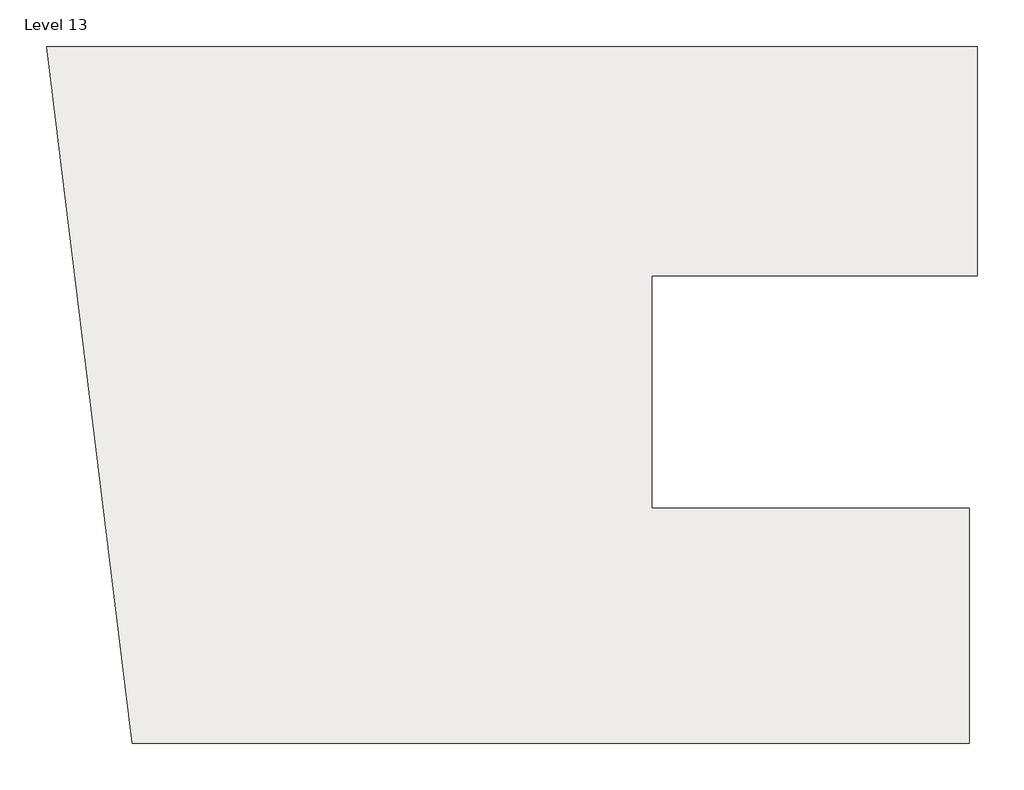
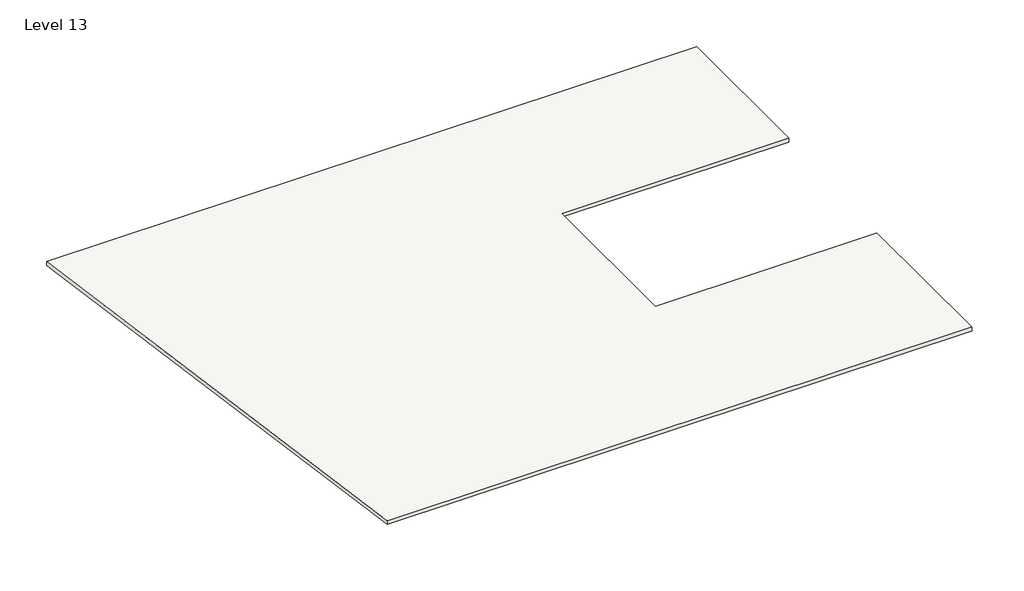
# One storey: 1 roof.
"""IFC4 building model written with IfcOpenShell, lengths in millimetres."""

from ifc_helpers import new_model, si_unit, frame, origin, place, context, project, spatial, polyline, outline, extrude, element, save

model = new_model("IFC4")

# Units and contexts
model_context = context("Model", 3, world=origin())
ifc_project = project(units=[si_unit("LENGTHUNIT", "METRE", prefix="MILLI")], contexts=[model_context])

# Site, building, storey
site = spatial("IfcSite", under=ifc_project)
building = spatial("IfcBuilding", under=site)
storey = spatial("IfcBuildingStorey", under=building, Name="Level 13", Elevation=36576.0)

# Roof
placement = place(None, origin())
element("IfcRoof", 1, ObjectType="Generic - 12\"", at=placement, inside=storey, context=model_context, shape_type="SweptSolid", body=[
    extrude(outline(polyline([(-8263.9071124, -7044.4846618), (-10506.1351996, 11216.9976508), (13902.5156363, 11216.9976508), (13902.5156363, 5212.8636295), (5368.1156363, 5212.8636295), (5368.1156363, -883.1363705), (13681.6928876, -883.1363705), (13681.6928876, -7044.4846618), (-8263.9071124, -7044.4846618)])), frame((0.0, 0.0, 36576.0), z_axis=(0.0, 0.0, 1.0), x_axis=(1.0, 0.0, 0.0)), (0.0, 0.0, 1.0), 152.4),
])

save(model, "model.ifc")

# Revit data of these elements
# Type "Generic - 12\""
#   Assembly Code = "B1020"
#   Layers, outside or top first: 0' - 6" no material (function 1)
# Element 1 (IfcRoof, "Generic - 12\"")
#   built-in parameter 1001705 = 120.5 (stored number, unit not read)
#   built-in parameter 1001710 = 33615
#   Phase Created = New Construction
#   Materials on its faces: "Default Roof"
# Materials
#   "Default Roof": colour RGB 88 101 114, transparency 0, Cost = 0
